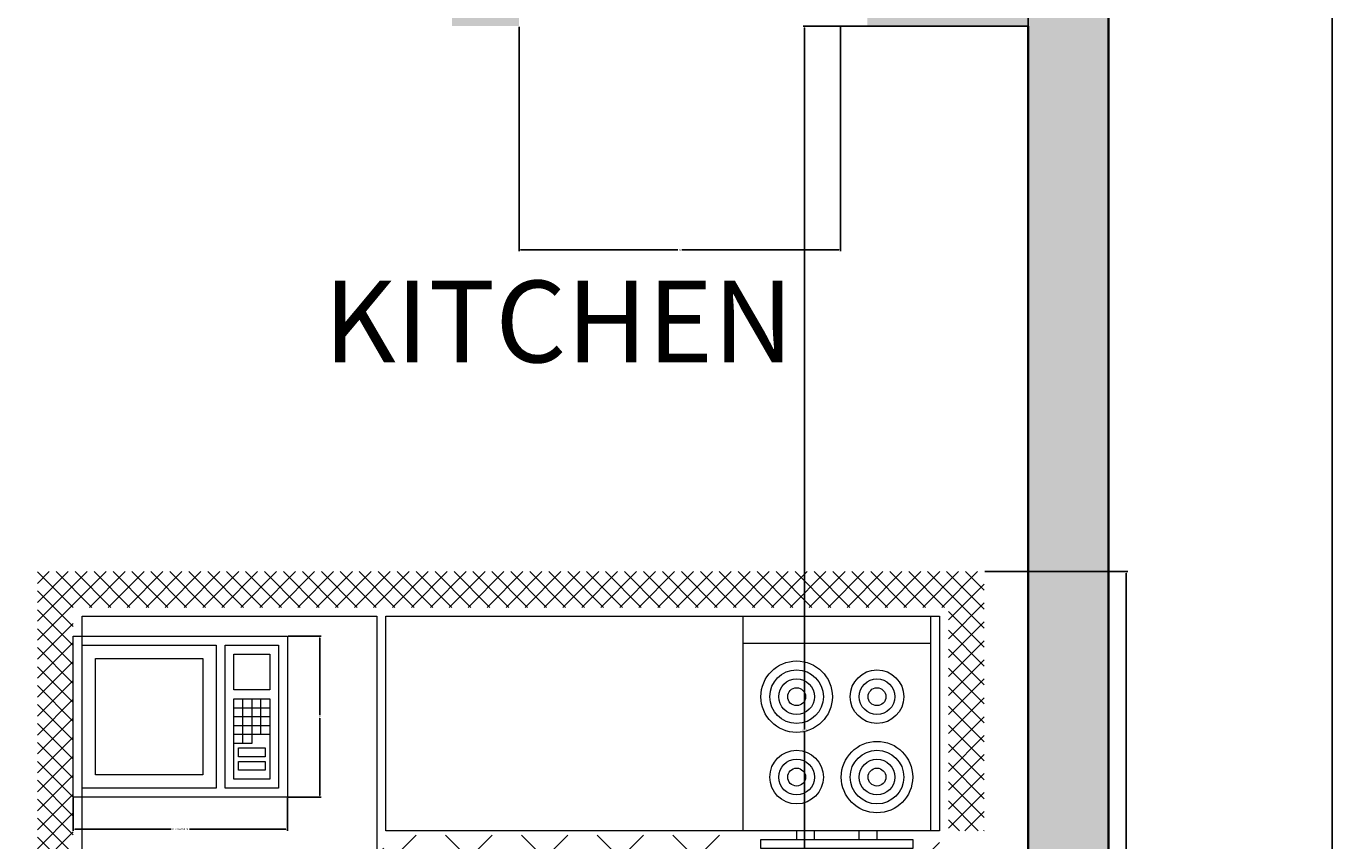
# Model space of a CAD drawing. Units: inches. Extents: x 1434 to 1845, y 1483 to 2014.
# Tile 7 of 11: x 1698 to 1845, y 1584 to 1675. Entities that reach past the tile are written whole.
import ezdxf

# ---------------------------------------------------------------- set-up
doc = ezdxf.new("R2010")
doc.units = ezdxf.units.IN
for name, color, linetype, lineweight in [('A-ANNO-DIMS', 2, 'Continuous', 18), ('A-AREA-IDEN', 7, 'Continuous', 25), ('A-EQPM', 9, 'Continuous', 18), ('A-FLOR-FIXT', 8, 'Continuous', 18), ('A-WALL', 7, 'Continuous', 35), ('A-WALL-PATT', 8, 'Continuous', 13)]:
    doc.layers.add(name, color=color, linetype=linetype, lineweight=lineweight)
doc.styles.get("Standard").update_dxf_attribs({"font": 'arial.ttf'})
doc.dimstyles.get("Standard").update_dxf_attribs({"dimtxt": 0.18, "dimasz": 0.18, "dimexe": 0.18, "dimexo": 0.0625, "dimgap": 0.09, "dimtad": 0, "dimtih": 1, "dimtoh": 1, "dimdec": 4, "dimzin": 0, "dimdsep": 46, "dimtxsty": 'Standard', "dimcen": 0.09, "dimadec": 0, "dimazin": 0, "dimtfac": 1, "dimtdec": 4, "dimtofl": 0, "dimtmove": 0, "dimatfit": 3, "dimfxl": 1, "dimtolj": 1, "dimtzin": 0, "dimarcsym": 0})

# ---------------------------------------------------------------- blocks, each defined once
blk = doc.blocks.new('Kitchen Layout - 7 x 8 ft')
for p, q in [((-5, 81.32), (2.68, 89)), ((-5, 83.44), (0.56, 89)), ((-5, 85.56), (-1.56, 89)), ((-5, 87.68), (-3.68, 89)), ((-1, 84.97), (-5, 88.97)), ((1.09, 85), (-2.91, 89)), ((3.21, 85), (-0.79, 89)), ((0.81, 85), (4.81, 89)), ((5.34, 85), (1.34, 89)), ((2.93, 85), (6.93, 89)), ((7.46, 85), (3.46, 89)), ((5.05, 85), (9.05, 89)), ((9.58, 85), (5.58, 89)), ((7.17, 85), (11.17, 89)), ((11.7, 85), (7.7, 89)), ((9.29, 85), (13.29, 89)), ((13.82, 85), (9.82, 89)), ((11.41, 85), (15.41, 89)), ((15.94, 85), (11.94, 89)), ((13.53, 85), (17.53, 89)), ((18.06, 85), (14.06, 89)), ((15.65, 85), (19.65, 89)), ((20.18, 85), (16.18, 89)), ((17.78, 85), (21.78, 89)), ((22.31, 85), (18.31, 89)), ((19.9, 85), (23.9, 89)), ((24.43, 85), (20.43, 89)), ((22.02, 85), (26.02, 89)), ((26.55, 85), (22.55, 89)), ((24.14, 85), (28.14, 89)), ((28.67, 85), (24.67, 89)), ((26.26, 85), (30.26, 89)), ((30.79, 85), (26.79, 89)), ((28.38, 85), (32.38, 89)), ((32.91, 85), (28.91, 89)), ((30.5, 85), (34.5, 89)), ((35.03, 85), (31.03, 89)), ((32.63, 85), (36.63, 89)), ((37.16, 85), (33.16, 89)), ((34.75, 85), (38.75, 89)), ((39.28, 85), (35.28, 89)), ((36.87, 85), (40.87, 89)), ((41.4, 85), (37.4, 89)), ((38.99, 85), (42.99, 89)), ((43.52, 85), (39.52, 89)), ((41.11, 85), (45.11, 89)), ((45.64, 85), (41.64, 89)), ((43.23, 85), (47.23, 89)), ((47.76, 85), (43.76, 89)), ((45.35, 85), (49.35, 89)), ((49.88, 85), (45.88, 89)), ((47.47, 85), (51.47, 89)), ((52, 85), (48, 89)), ((49.6, 85), (53.6, 89)), ((54.13, 85), (50.13, 89)), ((51.72, 85), (55.72, 89)), ((56.25, 85), (52.25, 89)), ((53.84, 85), (57.84, 89)), ((58.37, 85), (54.37, 89)), ((55.96, 85), (59.96, 89)), ((60.49, 85), (56.49, 89)), ((58.08, 85), (62.08, 89)), ((62.61, 85), (58.61, 89)), ((60.2, 85), (64.2, 89)), ((64.73, 85), (60.73, 89)), ((62.32, 85), (66.32, 89)), ((66.85, 85), (62.85, 89)), ((64.45, 85), (68.45, 89)), ((68.97, 85), (64.97, 89)), ((66.57, 85), (70.57, 89)), ((71.1, 85), (67.1, 89)), ((68.69, 85), (72.69, 89)), ((73.22, 85), (69.22, 89)), ((70.81, 85), (74.81, 89)), ((75.34, 85), (71.34, 89)), ((72.93, 85), (76.93, 89)), ((77.46, 85), (73.46, 89)), ((75.05, 85), (79.05, 89)), ((79.58, 85), (75.58, 89)), ((77.17, 85), (81.17, 89)), ((81.7, 85), (77.7, 89)), ((79.29, 85), (83.29, 89)), ((83.82, 85), (79.82, 89)), ((81.42, 85), (85.42, 89)), ((85.95, 85), (81.95, 89)), ((83.54, 85), (87.54, 89)), ((88.07, 85), (84.07, 89)), ((85.66, 85), (89.66, 89)), ((90.19, 85), (86.19, 89)), ((87.78, 85), (91.78, 89)), ((92.31, 85), (88.31, 89)), ((89.9, 85), (93.9, 89)), ((94.43, 85), (90.43, 89)), ((92.02, 85), (96.02, 89)), ((96.55, 85), (92.55, 89)), ((94.14, 85), (98.14, 89)), ((101, 82.67), (94.67, 89)), ((96.27, 85), (100.27, 89)), ((101, 84.79), (96.79, 89)), ((101, 86.92), (98.92, 89)), ((-1, 82.85), (-5, 86.85)), ((97, 83.61), (101, 87.61)), ((97, 81.49), (101, 85.49)), ((-1, 80.73), (-5, 84.73)), ((34, 84), (96, 84)), ((34, 60), (34, 84)), ((96, 84), (96, 60)), ((101, 80.55), (97, 84.55)), ((-5, 79.19), (-1, 83.19)), ((-1, 78.61), (-5, 82.61)), ((97, 79.37), (101, 83.37)), ((101, 78.43), (97, 82.43)), ((-5, 77.07), (-1, 81.07)), ((74, 81), (95, 81)), ((97, 77.25), (101, 81.25)), ((-1, 76.49), (-5, 80.49)), ((101, 76.31), (97, 80.31)), ((97, 75.13), (101, 79.13)), ((-5, 74.95), (-1, 78.95)), ((-1, 74.36), (-5, 78.36)), ((101, 74.19), (97, 78.19)), ((-5, 72.83), (-1, 76.83)), ((-1, 72.24), (-5, 76.24)), ((97, 73.01), (101, 77.01)), ((-5, 70.71), (-1, 74.71)), ((101, 72.07), (97, 76.07)), ((97, 70.89), (101, 74.89)), ((-1, 70.12), (-5, 74.12)), ((101, 69.95), (97, 73.95)), ((-5, 68.59), (-1, 72.59)), ((-1, 68), (-5, 72)), ((97, 68.76), (101, 72.76)), ((101, 67.82), (97, 71.82)), ((-5, 66.47), (-1, 70.47)), ((97, 66.64), (101, 70.64)), ((-1, 65.88), (-5, 69.88)), ((101, 65.7), (97, 69.7)), ((-5, 64.35), (-1, 68.35)), ((-1, 63.76), (-5, 67.76)), ((97, 64.52), (101, 68.52)), ((101, 63.58), (97, 67.58)), ((-5, 62.22), (-1, 66.22)), ((97, 62.4), (101, 66.4)), ((-1, 61.64), (-5, 65.64)), ((101, 61.46), (97, 65.46)), ((-5, 60.1), (-1, 64.1)), ((-1, 59.52), (-5, 63.52)), ((97, 60.28), (101, 64.28)), ((100.34, 60), (97, 63.34)), ((-5, 57.98), (-1, 61.98)), ((98.84, 60), (101, 62.16)), ((-1, 57.39), (-5, 61.39)), ((98.22, 60), (97, 61.22)), ((100.96, 60), (101, 60.04)), ((-1.73, 56), (-5, 59.27)), ((-4.86, 56), (-1, 59.86)), ((10.4, 24), (45.9, 59.5)), ((18.88, 24), (54.38, 59.5)), ((27.37, 24), (62.87, 59.5)), ((33.03, 55.11), (37.41, 59.5)), ((96, 60), (34, 60)), ((35.85, 24), (71.35, 59.5)), ((76.2, 24), (40.7, 59.5)), ((84.68, 24), (49.18, 59.5)), ((93.17, 24), (57.67, 59.5)), ((61.31, 24), (96, 58.69)), ((96, 29.65), (66.15, 59.5)), ((80, 60), (80, 59)), ((82, 59), (82, 60)), ((87, 59), (87, 60)), ((89, 60), (89, 59)), ((-3.85, 56), (-5, 57.15)), ((-2.74, 56), (-1, 57.74)), ((67.71, 24), (33.68, 58.04)), ((44.34, 24), (77.84, 57.5)), ((52.82, 24), (86.32, 57.5)), ((96, 38.14), (76.64, 57.5)), ((96, 46.63), (85.13, 57.5)), ((96, 55.11), (93.57, 57.54)), ((0, 57), (33, 57)), ((31, 55), (31, 56)), ((32, 56), (32, 55)), ((0, 30.57), (24.43, 55)), ((0, 39.06), (15.94, 55)), ((0, 47.54), (7.46, 55)), ((1.91, 24), (32.91, 55)), ((33.77, 24), (2.77, 55)), ((42.26, 24), (11.26, 55)), ((50.74, 24), (19.74, 55)), ((59.23, 24), (28.23, 55)), ((32, 55), (31, 55)), ((69.79, 24), (96, 50.21)), ((25.29, 24), (0, 49.29)), ((78.28, 24), (96, 41.72)), ((16.8, 24), (0, 40.8)), ((8.32, 24), (0, 32.32)), ((86.76, 24), (96, 33.24)), ((-5, 21.92), (-2.92, 24)), ((-5, 19.8), (-1, 23.8)), ((-1, 21.33), (-3.67, 24)), ((-1, 23.45), (-1.55, 24)), ((0, 24), (96, 24)), ((0, 0), (0, 24)), ((95.25, 24), (96, 24.75)), ((96, 24), (96, 0)), ((97, 22.1), (98.9, 24)), ((97, 19.97), (101, 23.97)), ((101, 21.16), (98.16, 24)), ((101, 23.28), (100.28, 24)), ((-1, 19.21), (-5, 23.21)), ((101, 19.03), (97, 23.03)), ((-5, 17.68), (-1, 21.68)), ((-1, 17.09), (-5, 21.09)), ((97, 17.85), (101, 21.85)), ((101, 16.91), (97, 20.91)), ((-5, 15.55), (-1, 19.55)), ((97, 15.73), (101, 19.73)), ((-1, 14.97), (-5, 18.97)), ((47.25, 6.5), (47.25, 18.5)), ((48.75, 18.5), (48.75, 6.5)), ((101, 14.79), (97, 18.79)), ((97, 13.61), (101, 17.61)), ((-5, 13.43), (-1, 17.43)), ((-1, 12.85), (-5, 16.85)), ((101, 12.67), (97, 16.67)), ((-5, 11.31), (-1, 15.31)), ((-1, 10.73), (-5, 14.73)), ((97, 11.49), (101, 15.49)), ((-5, 9.19), (-1, 13.19)), ((101, 10.55), (97, 14.55)), ((97, 9.37), (101, 13.37)), ((-1, 8.6), (-5, 12.6)), ((101, 8.43), (97, 12.43)), ((-5, 7.07), (-1, 11.07)), ((-1, 6.48), (-5, 10.48)), ((97, 7.25), (101, 11.25)), ((101, 6.31), (97, 10.31)), ((-5, 4.95), (-1, 8.95)), ((97, 5.12), (101, 9.12)), ((-1, 4.36), (-5, 8.36)), ((101, 4.18), (97, 8.18)), ((-5, 2.83), (-1, 6.83)), ((-1, 2.24), (-5, 6.24)), ((97, 3), (101, 7)), ((101, 2.06), (97, 6.06)), ((-5, 0.71), (-1, 4.71)), ((97, 0.88), (101, 4.88)), ((-1, 0.12), (-5, 4.12)), ((64, 4), (32, 4)), ((101, -0.06), (97, 3.94)), ((-5, -1.42), (-1, 2.58)), ((2, -5), (-5, 2)), ((93.24, -5), (101, 2.76)), ((101, -2.18), (97, 1.82)), ((-5, -3.54), (-1, 0.46)), ((96, 0), (0, 0)), ((95.36, -5), (101, 0.64)), ((-0.12, -5), (-5, -0.12)), ((-4.34, -5), (-0.34, -1)), ((-2.22, -5), (1.78, -1)), ((-0.1, -5), (3.9, -1)), ((4.12, -5), (0.12, -1)), ((2.02, -5), (6.02, -1)), ((6.24, -5), (2.24, -1)), ((4.14, -5), (8.14, -1)), ((8.36, -5), (4.36, -1)), ((6.27, -5), (10.27, -1)), ((10.48, -5), (6.48, -1)), ((8.39, -5), (12.39, -1)), ((12.6, -5), (8.6, -1)), ((10.51, -5), (14.51, -1)), ((14.73, -5), (10.73, -1)), ((12.63, -5), (16.63, -1)), ((16.85, -5), (12.85, -1)), ((14.75, -5), (18.75, -1)), ((18.97, -5), (14.97, -1)), ((16.87, -5), (20.87, -1)), ((21.09, -5), (17.09, -1)), ((18.99, -5), (22.99, -1)), ((23.21, -5), (19.21, -1)), ((21.11, -5), (25.11, -1)), ((25.33, -5), (21.33, -1)), ((23.24, -5), (27.24, -1)), ((27.45, -5), (23.45, -1)), ((25.36, -5), (29.36, -1)), ((29.57, -5), (25.57, -1)), ((30, -3.3), (27.7, -1)), ((30, -1.18), (29.82, -1)), ((66, -2.54), (67.54, -1)), ((66, -4.66), (69.66, -1)), ((69.88, -5), (66, -1.12)), ((67.78, -5), (71.78, -1)), ((72, -5), (68, -1)), ((69.9, -5), (73.9, -1)), ((74.12, -5), (70.12, -1)), ((72.03, -5), (76.03, -1)), ((76.24, -5), (72.24, -1)), ((74.15, -5), (78.15, -1)), ((78.36, -5), (74.36, -1)), ((76.27, -5), (80.27, -1)), ((80.49, -5), (76.49, -1)), ((78.39, -5), (82.39, -1)), ((82.61, -5), (78.61, -1)), ((80.51, -5), (84.51, -1)), ((84.73, -5), (80.73, -1)), ((82.63, -5), (86.63, -1)), ((86.85, -5), (82.85, -1)), ((84.75, -5), (88.75, -1)), ((88.97, -5), (84.97, -1)), ((86.88, -5), (90.88, -1)), ((91.09, -5), (87.09, -1)), ((89, -5), (93, -1)), ((93.21, -5), (89.21, -1)), ((91.12, -5), (95.12, -1)), ((95.34, -5), (91.34, -1)), ((97.46, -5), (93.46, -1)), ((99.58, -5), (95.58, -1)), ((101, -4.3), (97, -0.3)), ((-2.25, -5), (-5, -2.25)), ((27.48, -5), (30, -2.48)), ((97.48, -5), (101, -1.48)), ((-4.37, -5), (-5, -4.37)), ((67.76, -5), (66, -3.24)), ((99.6, -5), (101, -3.6)), ((29.6, -5), (30, -4.6))]:
    blk.add_line(p, q)
for points in [[(0, 56), (0, 84), (33, 84), (33, 56)], [(74, 60), (74, 84), (95, 84), (95, 60)], [(76, 58), (76, 59), (93, 59), (93, 58)]]:
    blk.add_lwpolyline(points, close=True)
for points in [[(33.5, 21), (62.5, 21)], [(32, 1.5), (32, 19.5)], [(34.5, 19.5), (46.25, 19.5)], [(49.75, 19.5), (61.5, 19.5)], [(64, 19.5), (64, 1.5)], [(33.5, 6.5), (33.5, 18.5)], [(62.5, 18.5), (62.5, 6.5)], [(46.25, 5.5), (34.5, 5.5)], [(61.5, 5.5), (49.75, 5.5)], [(62.5, 0), (33.5, 0)]]:
    blk.add_lwpolyline(points)
for centre, radius in [((80, 75), 4), ((80, 75), 3), ((89, 75), 3), ((80, 75), 2), ((89, 75), 2), ((80, 75), 1), ((89, 75), 1), ((80, 66), 3), ((89, 66), 4), ((89, 66), 3), ((80, 66), 2), ((89, 66), 2), ((80, 66), 1), ((89, 66), 1), ((40.5, 12.5), 1), ((55.5, 12.5), 1), ((40.5, 12.5), 0.5), ((55.5, 12.5), 0.5)]:
    blk.add_circle(centre, radius)
for centre, radius, start, end in [((33.5, 19.5), 1.5, 90, 180), ((62.5, 19.5), 1.5, 0, 90), ((34.5, 18.5), 1, 90, 180), ((46.25, 18.5), 1, 0, 90), ((49.75, 18.5), 1, 90, 180), ((61.5, 18.5), 1, 0, 90), ((34.5, 6.5), 1, 180, 270), ((46.25, 6.5), 1, 270, 0), ((49.75, 6.5), 1, 180, 270), ((61.5, 6.5), 1, 270, 0), ((33.5, 1.5), 1.5, 180, 270), ((62.5, 1.5), 1.5, 270, 0)]:
    blk.add_arc(centre, radius, start, end)
blk = doc.blocks.new('Microwave')
for p, q in [((19, 7), (19, 11)), ((20, 11), (20, 7)), ((21, 7), (21, 11)), ((18, 10), (22, 10)), ((22, 9), (18, 9)), ((18, 8), (22, 8)), ((22, 7), (18, 7)), ((20, 6), (18, 6)), ((19, 6), (19, 7)), ((20, 7), (20, 6))]:
    blk.add_line(p, q)
for points in [[(0, 0), (0, 18), (24, 18), (24, 0)], [(1, 1), (1, 17), (16, 17), (16, 1)], [(17, 1), (17, 17), (23, 17), (23, 1)], [(2.5, 2.5), (2.5, 15.5), (14.5, 15.5), (14.5, 2.5)], [(18, 12), (18, 16), (22, 16), (22, 12)], [(18, 2), (18, 11), (22, 11), (22, 2)], [(18.5, 4.5), (18.5, 5.5), (21.5, 5.5), (21.5, 4.5)], [(18.5, 3), (18.5, 4), (21.5, 4), (21.5, 3)]]:
    blk.add_lwpolyline(points, close=True)
blk = doc.blocks.new('*D47')
at = {"layer": 'A-ANNO-DIMS', "color": 0, "lineweight": -2, "transparency": 16777216}
for p, q in [((1805.61, 1614.02), (1821.63, 1614.02)), ((1821.45, 1613.84), (1821.45, 1567.2)), ((1821.45, 1520.2), (1821.45, 1566.84)), ((1805.61, 1520.02), (1821.63, 1520.02))]:
    blk.add_line(p, q, dxfattribs=at)
at = {"layer": 'A-ANNO-DIMS', "color": 0, "transparency": 16777216}
for points in [[(1821.42, 1613.84), (1821.48, 1613.84), (1821.45, 1614.02)], [(1821.42, 1520.2), (1821.48, 1520.2), (1821.45, 1520.02)]]:
    blk.add_solid(points, dxfattribs=at)
at = {"layer": 'Defpoints', "color": 0, "transparency": 16777216}
for p in [(1805.55, 1614.02), (1821.45, 1614.02), (1805.55, 1520.02)]:
    blk.add_point(p, dxfattribs=at)
at = {"layer": 'A-ANNO-DIMS', "color": 0, "transparency": 16777216, "insert": (1821.45, 1567.02), "char_height": 0.18, "attachment_point": 5}
blk.add_mtext('\\A1;94', dxfattribs=at)
blk = doc.blocks.new('*D48')
at = {"layer": 'A-ANNO-DIMS', "color": 0, "lineweight": -2, "transparency": 16777216}
for p, q in [((1703.55, 1588.71), (1703.55, 1585)), ((1727.55, 1588.71), (1727.55, 1585)), ((1703.73, 1585.18), (1714.51, 1585.18)), ((1727.37, 1585.18), (1716.59, 1585.18))]:
    blk.add_line(p, q, dxfattribs=at)
at = {"layer": 'A-ANNO-DIMS', "color": 0, "transparency": 16777216}
for points in [[(1703.73, 1585.21), (1703.73, 1585.15), (1703.55, 1585.18)], [(1727.37, 1585.21), (1727.37, 1585.15), (1727.55, 1585.18)]]:
    blk.add_solid(points, dxfattribs=at)
at = {"layer": 'Defpoints', "color": 0, "transparency": 16777216}
for p in [(1703.55, 1588.78), (1727.55, 1588.78), (1727.55, 1585.18)]:
    blk.add_point(p, dxfattribs=at)
at = {"layer": 'A-ANNO-DIMS', "color": 0, "transparency": 16777216, "insert": (1715.55, 1585.18), "char_height": 0.18, "attachment_point": 5}
blk.add_mtext('\\A1;MICROWAVE 24', dxfattribs=at)
blk = doc.blocks.new('*D49')
at = {"layer": 'A-ANNO-DIMS', "color": 0, "lineweight": -2, "transparency": 16777216}
for p, q in [((1727.61, 1606.78), (1731.33, 1606.78)), ((1731.15, 1606.6), (1731.15, 1597.96)), ((1731.15, 1588.96), (1731.15, 1597.6)), ((1727.61, 1588.78), (1731.33, 1588.78))]:
    blk.add_line(p, q, dxfattribs=at)
at = {"layer": 'A-ANNO-DIMS', "color": 0, "transparency": 16777216}
for points in [[(1731.12, 1606.6), (1731.18, 1606.6), (1731.15, 1606.78)], [(1731.12, 1588.96), (1731.18, 1588.96), (1731.15, 1588.78)]]:
    blk.add_solid(points, dxfattribs=at)
at = {"layer": 'Defpoints', "color": 0, "transparency": 16777216}
for p in [(1727.55, 1606.78), (1731.15, 1606.78), (1727.55, 1588.78)]:
    blk.add_point(p, dxfattribs=at)
at = {"layer": 'A-ANNO-DIMS', "color": 0, "transparency": 16777216, "insert": (1731.15, 1597.78), "char_height": 0.18, "attachment_point": 5}
blk.add_mtext('\\A1;18', dxfattribs=at)
blk = doc.blocks.new('*D55')
at = {"layer": 'A-ANNO-DIMS', "color": 0, "lineweight": -2, "transparency": 16777216}
for p, q in [((1819.54, 1988.36), (1844.68, 1988.36)), ((1844.5, 1988.18), (1844.5, 1748.54)), ((1844.5, 1508.54), (1844.5, 1748.17)), ((1819.54, 1508.36), (1844.68, 1508.36))]:
    blk.add_line(p, q, dxfattribs=at)
at = {"layer": 'A-ANNO-DIMS', "color": 0, "transparency": 16777216}
for points in [[(1844.47, 1988.18), (1844.53, 1988.18), (1844.5, 1988.36)], [(1844.47, 1508.54), (1844.53, 1508.54), (1844.5, 1508.36)]]:
    blk.add_solid(points, dxfattribs=at)
at = {"layer": 'Defpoints', "color": 0, "transparency": 16777216}
for p in [(1819.47, 1988.36), (1844.5, 1988.36), (1819.47, 1508.36)]:
    blk.add_point(p, dxfattribs=at)
at = {"layer": 'A-ANNO-DIMS', "color": 0, "transparency": 16777216, "insert": (1844.5, 1748.36), "char_height": 0.18, "attachment_point": 5}
blk.add_mtext('\\A1;480', dxfattribs=at)
blk = doc.blocks.new('*D58')
at = {"layer": 'A-ANNO-DIMS', "color": 0, "lineweight": -2, "transparency": 16777216}
for p, q in [((1670.97, 1974.79), (1670.97, 1483.15)), ((1810.47, 1974.79), (1810.47, 1483.15)), ((1671.15, 1483.33), (1740.34, 1483.33)), ((1810.29, 1483.33), (1741.11, 1483.33))]:
    blk.add_line(p, q, dxfattribs=at)
at = {"layer": 'A-ANNO-DIMS', "color": 0, "transparency": 16777216}
for points in [[(1671.15, 1483.36), (1671.15, 1483.3), (1670.97, 1483.33)], [(1810.29, 1483.36), (1810.29, 1483.3), (1810.47, 1483.33)]]:
    blk.add_solid(points, dxfattribs=at)
at = {"layer": 'Defpoints', "color": 0, "transparency": 16777216}
for p in [(1670.97, 1974.86), (1810.47, 1974.86), (1810.47, 1483.33)]:
    blk.add_point(p, dxfattribs=at)
at = {"layer": 'A-ANNO-DIMS', "color": 0, "transparency": 16777216, "insert": (1740.72, 1483.33), "char_height": 0.18, "attachment_point": 5}
blk.add_mtext('\\A1;139.5', dxfattribs=at)
blk = doc.blocks.new('*D67')
at = {"layer": 'A-ANNO-DIMS', "color": 0, "lineweight": -2, "transparency": 16777216}
for p, q in [((1694.97, 1517.42), (1694.97, 2013.56)), ((1695.15, 2013.38), (1752.34, 2013.38)), ((1810.29, 2013.38), (1753.11, 2013.38)), ((1810.47, 1517.42), (1810.47, 2013.56))]:
    blk.add_line(p, q, dxfattribs=at)
at = {"layer": 'A-ANNO-DIMS', "color": 0, "transparency": 16777216}
for points in [[(1695.15, 2013.41), (1695.15, 2013.35), (1694.97, 2013.38)], [(1810.29, 2013.41), (1810.29, 2013.35), (1810.47, 2013.38)]]:
    blk.add_solid(points, dxfattribs=at)
at = {"layer": 'Defpoints', "color": 0, "transparency": 16777216}
for p in [(1810.47, 2013.38), (1694.97, 1517.36), (1810.47, 1517.36)]:
    blk.add_point(p, dxfattribs=at)
at = {"layer": 'A-ANNO-DIMS', "color": 0, "transparency": 16777216, "insert": (1752.72, 2013.38), "char_height": 0.18, "attachment_point": 5}
blk.add_mtext('\\A1;115.5', dxfattribs=at)
blk = doc.blocks.new('*D85')
at = {"layer": 'A-ANNO-DIMS', "color": 0, "lineweight": -2, "transparency": 16777216}
for p, q in [((1810.41, 1675.08), (1785.27, 1675.08)), ((1785.45, 1674.9), (1785.45, 1596.4)), ((1785.45, 1517.54), (1785.45, 1596.04)), ((1810.41, 1517.36), (1785.27, 1517.36))]:
    blk.add_line(p, q, dxfattribs=at)
at = {"layer": 'A-ANNO-DIMS', "color": 0, "transparency": 16777216}
for points in [[(1785.42, 1674.9), (1785.48, 1674.9), (1785.45, 1675.08)], [(1785.42, 1517.54), (1785.48, 1517.54), (1785.45, 1517.36)]]:
    blk.add_solid(points, dxfattribs=at)
at = {"layer": 'Defpoints', "color": 0, "transparency": 16777216}
for p in [(1785.45, 1675.08), (1810.47, 1675.08), (1810.47, 1517.36)]:
    blk.add_point(p, dxfattribs=at)
at = {"layer": 'A-ANNO-DIMS', "color": 0, "transparency": 16777216, "insert": (1785.45, 1596.22), "char_height": 0.18, "attachment_point": 5}
blk.add_mtext('\\A1;157.73', dxfattribs=at)
blk = doc.blocks.new('*D91')
at = {"layer": 'A-ANNO-DIMS', "color": 0, "lineweight": -2, "transparency": 16777216}
for p, q in [((1753.47, 1675.02), (1753.47, 1649.88)), ((1789.47, 1675.02), (1789.47, 1649.88)), ((1753.65, 1650.06), (1771.26, 1650.06)), ((1789.29, 1650.06), (1771.69, 1650.06))]:
    blk.add_line(p, q, dxfattribs=at)
at = {"layer": 'A-ANNO-DIMS', "color": 0, "transparency": 16777216}
for points in [[(1753.65, 1650.09), (1753.65, 1650.03), (1753.47, 1650.06)], [(1789.29, 1650.09), (1789.29, 1650.03), (1789.47, 1650.06)]]:
    blk.add_solid(points, dxfattribs=at)
at = {"layer": 'Defpoints', "color": 0, "transparency": 16777216}
for p in [(1753.47, 1675.08), (1789.47, 1675.08), (1753.47, 1650.06)]:
    blk.add_point(p, dxfattribs=at)
at = {"layer": 'A-ANNO-DIMS', "color": 0, "transparency": 16777216, "insert": (1771.47, 1650.06), "char_height": 0.18, "attachment_point": 5}
blk.add_mtext('\\A1;36', dxfattribs=at)

msp = doc.modelspace()

# ---------------------------------------------------------------- hatches: boundary and pattern name
at = {"layer": 'A-WALL-PATT'}
h = msp.add_hatch(color=256, dxfattribs=at)
h.dxf.hatch_style = 1
h.paths.add_polyline_path([(1472.9742, 1730.3553), (1577.9742, 1730.3553), (1577.9742, 1734.8553), (1573.4742, 1734.8553), (1573.4742, 1815.8553), (1568.9742, 1815.8553), (1568.9742, 1734.8553), (1472.9742, 1734.8553), (1472.9742, 1770.1951), (1459.9742, 1770.1951), (1459.9742, 1782.1951), (1459.9742, 1818.1951), (1472.9742, 1818.1951), (1472.9742, 1854.8553), (1568.9742, 1854.8553), (1568.9742, 1851.8553), (1573.4742, 1851.8553), (1573.4742, 1854.8553), (1573.4742, 1859.3553), (1472.9742, 1859.3553), (1472.9742, 1899.9369), (1459.9742, 1899.9369), (1459.9742, 1911.9369), (1459.9742, 1947.9369), (1472.9742, 1947.9369), (1472.9742, 1974.8553), (1513.9785, 1974.8553), (1513.9785, 1987.8553), (1561.9785, 1987.8553), (1561.9785, 1974.8553), (1612.4742, 1974.8553), (1612.4742, 1859.3553), (1609.4742, 1859.3553), (1609.4742, 1854.8553), (1616.9742, 1854.8553), (1616.9742, 1910.3553), (1625.153, 1910.3553), (1625.153, 1914.8553), (1616.9742, 1914.8553), (1616.9742, 1988.3553), (1459.4742, 1988.3553), (1459.4742, 1508.3553), (1630.4742, 1508.3553), (1630.4742, 1517.3553), (1472.9742, 1517.3553), (1472.9742, 1586.3553), (1616.9742, 1586.3553), (1616.9742, 1583.3553), (1621.4742, 1583.3553), (1621.4742, 1586.3553), (1621.4742, 1734.8553), (1616.9742, 1734.8553), (1613.9742, 1734.8553), (1613.9742, 1730.3553), (1616.9742, 1730.3553), (1616.9742, 1590.8553), (1472.9742, 1590.8553), (1472.9742, 1635.7299), (1459.9742, 1635.7299), (1459.9742, 1647.7299), (1459.9742, 1683.7299), (1472.9742, 1683.7299)])
h.paths.add_polyline_path([(1819.4742, 1773.1667), (1810.4742, 1773.1667), (1810.4742, 1734.8553), (1714.4742, 1734.8553), (1714.4742, 1815.8553), (1709.9742, 1815.8553), (1709.9742, 1730.3553), (1745.9742, 1730.3553), (1745.9742, 1675.0848), (1753.4742, 1675.0848), (1753.4742, 1679.5848), (1750.4742, 1679.5848), (1750.4742, 1730.3553), (1810.4742, 1730.3553), (1810.4742, 1679.5848), (1792.4742, 1679.5848), (1792.4742, 1675.0848), (1810.4742, 1675.0848), (1810.4742, 1517.3553), (1775.1129, 1517.3553), (1775.1129, 1508.3553), (1819.4742, 1508.3553)])
h.paths.add_polyline_path([(1739.1129, 1517.3553), (1694.9742, 1517.3553), (1694.9742, 1730.3553), (1690.4742, 1730.3553), (1690.4742, 1517.3553), (1678.4742, 1517.3553), (1675.4742, 1517.3553), (1672.8212, 1517.3553), (1672.8212, 1508.3553), (1678.4742, 1508.3553), (1739.1129, 1508.3553)])
h.paths.add_polyline_path([(1735.6549, 1987.8553), (1783.6549, 1987.8553), (1783.6549, 1974.8553), (1810.4742, 1974.8553), (1810.4742, 1859.3553), (1709.9742, 1859.3553), (1709.9742, 1854.8553), (1709.9742, 1851.8553), (1714.4742, 1851.8553), (1714.4742, 1854.8553), (1810.4742, 1854.8553), (1810.4742, 1809.1667), (1819.4742, 1809.1667), (1819.4742, 1988.3553), (1666.4742, 1988.3553), (1666.4742, 1914.8553), (1661.1087, 1914.8553), (1661.1087, 1910.3553), (1666.4742, 1910.3553), (1666.4742, 1854.8553), (1673.9742, 1854.8553), (1673.9742, 1859.3553), (1670.9742, 1859.3553), (1670.9742, 1974.8553), (1735.6549, 1974.8553)])

# ---------------------------------------------------------------- linework, layer by layer
at = {"layer": 'A-WALL'}
msp.add_line((1810.4742, 1517.3553), (1810.4742, 1675.0848), dxfattribs=at)
msp.add_lwpolyline([(1678.4742, 1508.3553), (1819.4742, 1508.3553), (1819.4742, 1988.3553), (1459.4742, 1988.3553), (1459.4742, 1508.3553), (1630.4742, 1508.3553)], dxfattribs=at)

# ---------------------------------------------------------------- block references
at = {"layer": 'A-EQPM'}
msp.add_blockref('Microwave', (1703.5505, 1588.7773), dxfattribs=at)
at = {"layer": 'A-FLOR-FIXT'}
msp.add_blockref('Kitchen Layout - 7 x 8 ft', (1704.5505, 1525.0191), dxfattribs=at)

# ---------------------------------------------------------------- texts
at = {"layer": 'A-AREA-IDEN'}
msp.add_text('KITCHEN ', height=9.14668, dxfattribs=at).set_placement((1731.62, 1637.4459))

# ---------------------------------------------------------------- dimensions: what is measured, and where the dimension line sits
at = {"layer": 'A-ANNO-DIMS'}
for base, p1, p2, picture, middle in [((1810.4742, 2013.3803), (1694.9742, 1517.3553), (1810.4742, 1517.3553), '*D67', (1752.7242, 2013.3803)), ((1810.4742, 1483.3303), (1670.9742, 1974.8553), (1810.4742, 1974.8553), '*D58', (1740.7242, 1483.3303))]:
    dim = msp.add_linear_dim(base=base, p1=p1, p2=p2, dimstyle='Standard', override={"dimdec": 1, "dimlfac": 1, "dimrnd": 0, "dimzin": 0, "dimdsep": 46, "dimlunit": 2}, dxfattribs=at)
    dim.commit()
    dim.dimension.update_dxf_attribs({"geometry": picture, "text_midpoint": middle})
for base, p1, p2, angle, override, picture, middle in [((1844.4992, 1988.3553), (1819.4742, 1508.3553), (1819.4742, 1988.3553), 90, {"dimdec": 0, "dimlfac": 1, "dimrnd": 0, "dimzin": 0, "dimdsep": 46, "dimlunit": 2}, '*D55', (1844.4992, 1748.3553)), ((1753.4742, 1650.0598), (1789.4742, 1675.0848), (1753.4742, 1675.0848), 180, {"dimdec": 0, "dimlfac": 1, "dimrnd": 0, "dimzin": 0, "dimdsep": 46, "dimlunit": 2}, '*D91', (1771.4742, 1650.0598)), ((1785.4492, 1675.0848), (1810.4742, 1517.3553), (1810.4742, 1675.0848), 90, {"dimdec": 2, "dimlfac": 1, "dimrnd": 0, "dimzin": 0, "dimdsep": 46, "dimlunit": 2}, '*D85', (1785.4492, 1596.2201)), ((1821.4505, 1614.0191), (1805.5505, 1520.0191), (1805.5505, 1614.0191), 90, {"dimdec": 0, "dimlfac": 1, "dimrnd": 0, "dimzin": 0, "dimdsep": 46, "dimlunit": 2}, '*D47', (1821.4505, 1567.0191)), ((1731.1505, 1606.7773), (1727.5505, 1588.7773), (1727.5505, 1606.7773), 90, {"dimdec": 0, "dimlfac": 1, "dimrnd": 0, "dimzin": 0, "dimdsep": 46, "dimlunit": 2}, '*D49', (1731.1505, 1597.7773))]:
    dim = msp.add_linear_dim(base=base, p1=p1, p2=p2, angle=angle, dimstyle='Standard', override=override, dxfattribs=at)
    dim.commit()
    dim.dimension.update_dxf_attribs({"geometry": picture, "text_midpoint": middle})
dim = msp.add_linear_dim(base=(1727.5505, 1585.1773), p1=(1703.5505, 1588.7773), p2=(1727.5505, 1588.7773), text='MICROWAVE <>', dimstyle='Standard', override={"dimdec": 0, "dimlfac": 1, "dimrnd": 0, "dimzin": 0, "dimdsep": 46, "dimlunit": 2}, dxfattribs=at)
dim.commit()
dim.dimension.update_dxf_attribs({"geometry": '*D48', "text_midpoint": (1715.5505, 1585.1773)})

doc.saveas('drawing.dxf')
